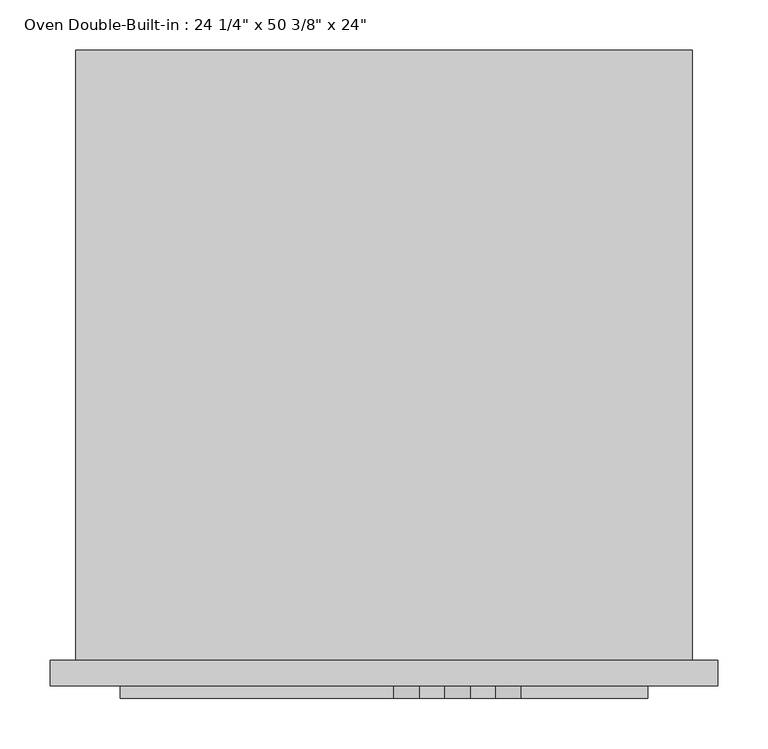
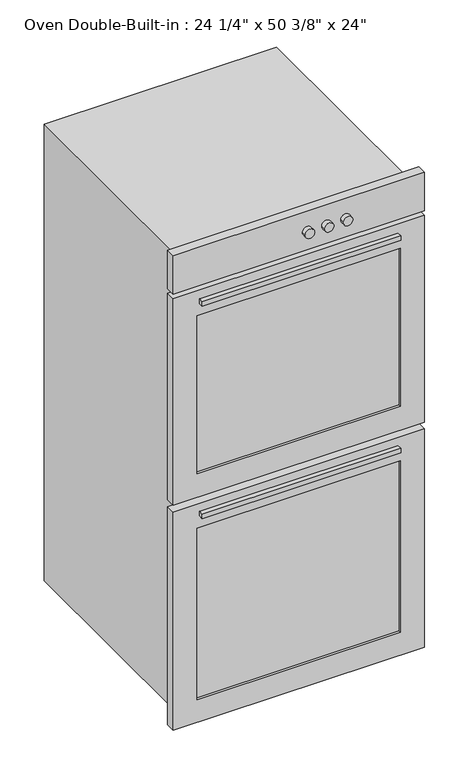
"""IFC4 building model written with IfcOpenShell, lengths in millimetres: proxy geometry."""

from ifc_helpers import new_model, si_unit, point, frame, frame_2d, origin, place, context, project, spatial, polyline, circle_curve, trimmed, segment, composite_curve, outline, extrude, source, transform, mapped, element, save


def proxy_f893816d(model_context):
    return source(origin(), model_context, "Body", "SweptSolid", [
        extrude(outline(polyline([(247.4000727, -138.3341411), (-317.7499273, -138.3341411), (-317.7499273, 420.4658589), (247.4000727, 420.4658589), (247.4000727, -138.3341411)])), frame((0.0, 0.0, 941.3875), z_axis=(0.0, 0.0, 1.0), x_axis=(1.0, 0.0, 0.0)), (0.0, 0.0, 1.0), 19.05),
        extrude(outline(polyline([(247.4000727, -163.7341411), (-317.7499273, -163.7341411), (-317.7499273, -138.3341411), (247.4000727, -138.3341411), (247.4000727, -163.7341411)])), frame((0.0, 0.0, 1514.5470137), z_axis=(0.0, 0.0, 1.0), x_axis=(1.0, 0.0, 0.0)), (0.0, 0.0, 1.0), 95.1779863),
        extrude(outline(polyline([(247.4000727, -163.7341411), (-317.7499273, -163.7341411), (-317.7499273, -138.3341411), (247.4000727, -138.3341411), (247.4000727, -163.7341411)])), frame((0.0, 0.0, 909.6375), z_axis=(0.0, 0.0, 1.0), x_axis=(1.0, 0.0, 0.0)), (0.0, 0.0, 1.0), 82.55),
        extrude(outline(composite_curve([segment(trimmed(circle_curve(frame_2d((1604.846693, -12.6998447)), 12.7), [point((1604.846693, -25.3998447))], [point((1604.846693, 0.0001553))], False, "CARTESIAN"), True, "CONTINUOUS"), segment(trimmed(circle_curve(frame_2d((1604.846693, -12.6998447)), 12.7), [point((1604.846693, 0.0001553))], [point((1604.846693, -25.3998447))], False, "CARTESIAN"), True, "CONTINUOUS")], self_intersect=False)), frame((0.0, -201.8341411, 0.0), z_axis=(0.0, 1.0, 0.0), x_axis=(0.0, 0.0, 1.0)), (0.0, 0.0, 1.0), 12.7),
        extrude(outline(composite_curve([segment(trimmed(circle_curve(frame_2d((1604.846693, 38.1001553)), 12.7), [point((1604.846693, 25.4001553))], [point((1604.846693, 50.8001553))], False, "CARTESIAN"), True, "CONTINUOUS"), segment(trimmed(circle_curve(frame_2d((1604.846693, 38.1001553)), 12.7), [point((1604.846693, 50.8001553))], [point((1604.846693, 25.4001553))], False, "CARTESIAN"), True, "CONTINUOUS")], self_intersect=False)), frame((0.0, -201.8341411, 0.0), z_axis=(0.0, 1.0, 0.0), x_axis=(0.0, 0.0, 1.0)), (0.0, 0.0, 1.0), 12.7),
        extrude(outline(composite_curve([segment(trimmed(circle_curve(frame_2d((1604.846693, 88.9001553)), 12.7), [point((1604.846693, 76.2001553))], [point((1604.846693, 101.6001553))], False, "CARTESIAN"), True, "CONTINUOUS"), segment(trimmed(circle_curve(frame_2d((1604.846693, 88.9001553)), 12.7), [point((1604.846693, 101.6001553))], [point((1604.846693, 76.2001553))], False, "CARTESIAN"), True, "CONTINUOUS")], self_intersect=False)), frame((0.0, -201.8341411, 0.0), z_axis=(0.0, 1.0, 0.0), x_axis=(0.0, 0.0, 1.0)), (0.0, 0.0, 1.0), 12.7),
        extrude(outline(polyline([(228.3500727, -201.8341411), (-298.6999273, -201.8341411), (-298.6999273, -189.1341411), (228.3500727, -189.1341411), (228.3500727, -201.8341411)])), frame((0.0, 0.0, 1501.8470137), z_axis=(0.0, 0.0, 1.0), x_axis=(1.0, 0.0, 0.0)), (0.0, 0.0, 1.0), 12.7),
        extrude(outline(polyline([(228.3500727, -201.8341411), (-298.6999273, -201.8341411), (-298.6999273, -189.1341411), (228.3500727, -189.1341411), (228.3500727, -201.8341411)])), frame((0.0, 0.0, 906.5345137), z_axis=(0.0, 0.0, 1.0), x_axis=(1.0, 0.0, 0.0)), (0.0, 0.0, 1.0), 12.7),
        extrude(outline(polyline([(234.7000727, -182.7841411), (-305.0499273, -182.7841411), (-305.0499273, -176.4341411), (234.7000727, -176.4341411), (234.7000727, -182.7841411)])), frame((0.0, 0.0, 1027.1125), z_axis=(0.0, 0.0, 1.0), x_axis=(1.0, 0.0, 0.0)), (0.0, 0.0, 1.0), 442.9125),
        extrude(outline(polyline([(234.7000727, -182.7841411), (-305.0499273, -182.7841411), (-305.0499273, -176.4341411), (234.7000727, -176.4341411), (234.7000727, -182.7841411)])), frame((0.0, 0.0, 393.7), z_axis=(0.0, 0.0, 1.0), x_axis=(1.0, 0.0, 0.0)), (0.0, 0.0, 1.0), 481.0125),
        extrude(outline(polyline([(298.2000727, -189.1341411), (-368.5499273, -189.1341411), (-368.5499273, -163.7341411), (298.2000727, -163.7341411), (298.2000727, -189.1341411)])), frame((0.0, 0.0, 1552.575), z_axis=(0.0, 0.0, 1.0), x_axis=(1.0, 0.0, 0.0)), (0.0, 0.0, 1.0), 107.95),
        extrude(outline(polyline([(1539.875, 298.2000727), (1539.875, -368.5499273), (960.4375, -368.5499273), (960.4375, 298.2000727), (1539.875, 298.2000727)]), holes=[polyline([(1470.025, 234.7000727), (1027.1125, 234.7000727), (1027.1125, -305.0499273), (1470.025, -305.0499273), (1470.025, 234.7000727)])]), frame((0.0, -189.1341411, 0.0), z_axis=(0.0, 1.0, 0.0), x_axis=(0.0, 0.0, 1.0)), (0.0, 0.0, 1.0), 25.4),
        extrude(outline(polyline([(941.3875, 298.2000727), (941.3875, -368.5499273), (330.2, -368.5499273), (330.2, 298.2000727), (941.3875, 298.2000727)]), holes=[polyline([(874.7125, 234.7000727), (393.7, 234.7000727), (393.7, -305.0499273), (874.7125, -305.0499273), (874.7125, 234.7000727)])]), frame((0.0, -189.1341411, 0.0), z_axis=(0.0, 1.0, 0.0), x_axis=(0.0, 0.0, 1.0)), (0.0, 0.0, 1.0), 25.4),
        extrude(outline(polyline([(247.4000727, 420.4658589), (-317.7499273, 420.4658589), (-317.7499273, 445.8658589), (247.4000727, 445.8658589), (247.4000727, 420.4658589)])), frame((0.0, 0.0, 381.0), z_axis=(0.0, 0.0, 1.0), x_axis=(1.0, 0.0, 0.0)), (0.0, 0.0, 1.0), 1228.725),
        extrude(outline(polyline([(1635.125, 272.8000727), (1635.125, -343.1499273), (355.6, -343.1499273), (355.6, 272.8000727), (1635.125, 272.8000727)]), holes=[polyline([(1609.725, 247.4000727), (381.0, 247.4000727), (381.0, -317.7499273), (1609.725, -317.7499273), (1609.725, 247.4000727)])]), frame((0.0, -163.7341411, 0.0), z_axis=(0.0, 1.0, 0.0), x_axis=(0.0, 0.0, 1.0)), (0.0, 0.0, 1.0), 609.6),
    ])


if __name__ == "__main__":
    model = new_model("IFC4")
    model_context = context("Model", 3, world=origin())
    ifc_project = project(units=[si_unit("LENGTHUNIT", "METRE", prefix="MILLI")], contexts=[model_context])
    site = spatial("IfcSite", under=ifc_project)
    building = spatial("IfcBuilding", under=site)
    placement = place(None, origin())
    proxy_shape = proxy_f893816d(model_context)
    element("IfcBuildingElementProxy", 1, Name="Oven Double-Built-in : 24 1/4\" x 50 3/8\" x 24\"", ObjectType="Oven Double-Built-in : 24 1/4\" x 50 3/8\" x 24\"", at=placement, inside=building, context=model_context, shape_type="MappedRepresentation", body=[
        mapped(proxy_shape, transform((0.0, 0.0, 0.0), x_axis=(1.0, 0.0, 0.0), y_axis=(0.0, 1.0, 0.0), z_axis=(0.0, 0.0, 1.0))),
    ])
    save(model, "model.ifc")

# Revit data of these elements
# Type "Oven Double-Built-in : 24 1/4\" x 50 3/8\" x 24\""
#   Label = "OVEN"
#   Assembly Code = "E1090400"
#   Depth = 2' - 0"
#   Height = 4' - 2 3/8"
#   Width = 2' - 0 1/4"
#   Oven Material = Metal - Stainless Steel, Polished
#   Default Elevation = 0
# Element 1 (IfcBuildingElementProxy, "Oven Double-Built-in : 24 1/4\" x 50 3/8\" x 24\"")
#   Materials on its faces: "Steel", "Metal - Stainless Steel, Polished", "Glass"
# Materials
#   "Metal - Stainless Steel, Polished": class "Metal", colour RGB 216 216 216, transparency 0
#   "Steel": class "Metal", colour RGB 247 247 247, transparency 0, Description = "Steel, mill finish", Cost = 0
#   "Glass": class "Glass", colour RGB 0 128 192, transparency 0.75, Description = "Soda Lime Glass", Cost = 0
